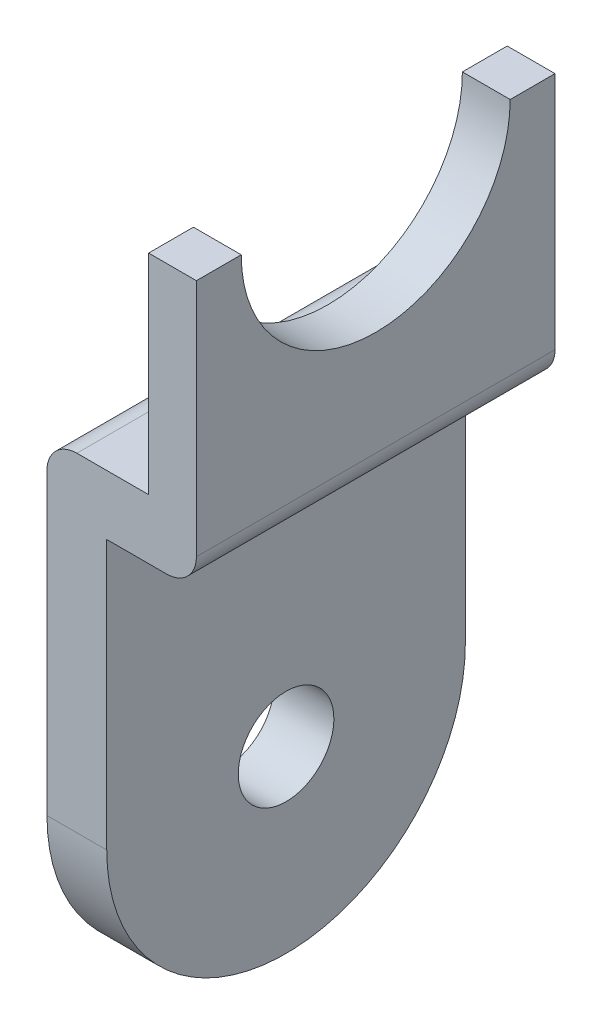
ISO-10303-21;
HEADER;
FILE_DESCRIPTION(('STEP AP214'),'2;1');
FILE_NAME('part.step','',(''),(''),'','','');
FILE_SCHEMA(('AUTOMOTIVE_DESIGN { 1 0 10303 214 1 1 1 1 }'));
ENDSEC;
DATA;
#1=APPLICATION_CONTEXT('core data for automotive mechanical design processes');
#2=APPLICATION_PROTOCOL_DEFINITION('international standard','automotive_design',2000,#1);
#3=PRODUCT_CONTEXT('',#1,'mechanical');
#4=PRODUCT('Part','Part','',(#3));
#5=PRODUCT_RELATED_PRODUCT_CATEGORY('part','',(#4));
#6=PRODUCT_DEFINITION_FORMATION('','',#4);
#7=PRODUCT_DEFINITION_CONTEXT('part definition',#1,'design');
#8=PRODUCT_DEFINITION('design','',#6,#7);
#9=PRODUCT_DEFINITION_SHAPE('','',#8);
#10=(LENGTH_UNIT() NAMED_UNIT(*) SI_UNIT(.MILLI.,.METRE.));
#11=(NAMED_UNIT(*) PLANE_ANGLE_UNIT() SI_UNIT($,.RADIAN.));
#12=(NAMED_UNIT(*) SI_UNIT($,.STERADIAN.) SOLID_ANGLE_UNIT());
#13=UNCERTAINTY_MEASURE_WITH_UNIT(LENGTH_MEASURE(1.E-05),#10,'distance_accuracy_value','');
#14=(GEOMETRIC_REPRESENTATION_CONTEXT(3) GLOBAL_UNCERTAINTY_ASSIGNED_CONTEXT((#13)) GLOBAL_UNIT_ASSIGNED_CONTEXT((#10,
#11,#12)) REPRESENTATION_CONTEXT('',''));
#15=CARTESIAN_POINT('',(0.,0.,0.));
#16=DIRECTION('',(0.,0.,1.));
#17=DIRECTION('',(1.,0.,0.));
#18=AXIS2_PLACEMENT_3D('',#15,#16,#17);
#19=CARTESIAN_POINT('',(3.4,7.,6.));
#20=DIRECTION('',(0.,-1.,0.));
#21=DIRECTION('',(0.,0.,-1.));
#22=AXIS2_PLACEMENT_3D('',#19,#20,#21);
#23=PLANE('',#22);
#24=DIRECTION('',(0.,0.,-1.));
#25=VECTOR('',#24,1.);
#26=CARTESIAN_POINT('',(3.4,7.,6.));
#27=LINE('',#26,#25);
#28=CARTESIAN_POINT('',(3.4,7.,-4.5));
#29=VERTEX_POINT('',#28);
#30=CARTESIAN_POINT('',(3.4,7.,-6.));
#31=VERTEX_POINT('',#30);
#32=EDGE_CURVE('E147',#29,#31,#27,.T.);
#33=ORIENTED_EDGE('',*,*,#32,.F.);
#34=DIRECTION('',(1.,0.,0.));
#35=VECTOR('',#34,1.);
#36=CARTESIAN_POINT('',(-0.00100000000000013,7.,-4.5));
#37=LINE('',#36,#35);
#38=CARTESIAN_POINT('',(5.,7.,-4.5));
#39=VERTEX_POINT('',#38);
#40=EDGE_CURVE('E128',#29,#39,#37,.T.);
#41=ORIENTED_EDGE('',*,*,#40,.T.);
#42=DIRECTION('',(0.,0.,-1.));
#43=VECTOR('',#42,1.);
#44=CARTESIAN_POINT('',(5.,7.,6.));
#45=LINE('',#44,#43);
#46=CARTESIAN_POINT('',(5.,7.,-6.));
#47=VERTEX_POINT('',#46);
#48=EDGE_CURVE('E144',#39,#47,#45,.T.);
#49=ORIENTED_EDGE('',*,*,#48,.T.);
#50=DIRECTION('',(-1.,0.,0.));
#51=VECTOR('',#50,1.);
#52=CARTESIAN_POINT('',(3.4,7.,-6.));
#53=LINE('',#52,#51);
#54=EDGE_CURVE('E216',#47,#31,#53,.T.);
#55=ORIENTED_EDGE('',*,*,#54,.T.);
#56=EDGE_LOOP('',(#33,#41,#49,#55));
#57=FACE_BOUND('',#56,.T.);
#58=ADVANCED_FACE('F39',(#57),#23,.F.);
#59=CARTESIAN_POINT('',(2.,-2.,6.));
#60=DIRECTION('',(-1.,0.,0.));
#61=DIRECTION('',(0.,-1.,0.));
#62=AXIS2_PLACEMENT_3D('',#59,#60,#61);
#63=PLANE('',#62);
#64=CARTESIAN_POINT('',(2.,-11.,0.));
#65=DIRECTION('',(1.,0.,0.));
#66=DIRECTION('',(0.,1.,0.));
#67=AXIS2_PLACEMENT_3D('',#64,#65,#66);
#68=CIRCLE('',#67,1.6);
#69=CARTESIAN_POINT('',(2.,-9.4,0.));
#70=VERTEX_POINT('',#69);
#71=EDGE_CURVE('E280',#70,#70,#68,.T.);
#72=ORIENTED_EDGE('',*,*,#71,.F.);
#73=EDGE_LOOP('',(#72));
#74=FACE_BOUND('',#73,.T.);
#75=DIRECTION('',(0.,1.,0.));
#76=VECTOR('',#75,1.);
#77=CARTESIAN_POINT('',(2.,-2.,6.));
#78=LINE('',#77,#76);
#79=CARTESIAN_POINT('',(2.,-11.,6.));
#80=VERTEX_POINT('',#79);
#81=CARTESIAN_POINT('',(2.,-2.,6.));
#82=VERTEX_POINT('',#81);
#83=EDGE_CURVE('E194',#80,#82,#78,.T.);
#84=ORIENTED_EDGE('',*,*,#83,.F.);
#85=CARTESIAN_POINT('',(2.,-11.,0.));
#86=DIRECTION('',(1.,0.,0.));
#87=DIRECTION('',(0.,1.,0.));
#88=AXIS2_PLACEMENT_3D('',#85,#86,#87);
#89=CIRCLE('',#88,6.);
#90=CARTESIAN_POINT('',(2.,-11.,-6.));
#91=VERTEX_POINT('',#90);
#92=EDGE_CURVE('E265',#80,#91,#89,.T.);
#93=ORIENTED_EDGE('',*,*,#92,.T.);
#94=DIRECTION('',(0.,1.,0.));
#95=VECTOR('',#94,1.);
#96=CARTESIAN_POINT('',(2.,-2.,-6.));
#97=LINE('',#96,#95);
#98=CARTESIAN_POINT('',(2.,-2.,-6.));
#99=VERTEX_POINT('',#98);
#100=EDGE_CURVE('E209',#91,#99,#97,.T.);
#101=ORIENTED_EDGE('',*,*,#100,.T.);
#102=DIRECTION('',(0.,0.,-1.));
#103=VECTOR('',#102,1.);
#104=CARTESIAN_POINT('',(2.,-2.,6.));
#105=LINE('',#104,#103);
#106=EDGE_CURVE('E156',#82,#99,#105,.T.);
#107=ORIENTED_EDGE('',*,*,#106,.F.);
#108=EDGE_LOOP('',(#84,#93,#101,#107));
#109=FACE_BOUND('',#108,.T.);
#110=ADVANCED_FACE('F229',(#74,#109),#63,.F.);
#111=CARTESIAN_POINT('',(5.,-2.,6.));
#112=DIRECTION('',(0.,1.,0.));
#113=DIRECTION('',(-1.,0.,0.));
#114=AXIS2_PLACEMENT_3D('',#111,#112,#113);
#115=PLANE('',#114);
#116=DIRECTION('',(1.,0.,0.));
#117=VECTOR('',#116,1.);
#118=CARTESIAN_POINT('',(5.,-2.,-6.));
#119=LINE('',#118,#117);
#120=CARTESIAN_POINT('',(4.,-2.,-6.));
#121=VERTEX_POINT('',#120);
#122=EDGE_CURVE('E215',#99,#121,#119,.T.);
#123=ORIENTED_EDGE('',*,*,#122,.T.);
#124=DIRECTION('',(0.,0.,-1.));
#125=VECTOR('',#124,1.);
#126=CARTESIAN_POINT('',(4.,-2.,6.));
#127=LINE('',#126,#125);
#128=CARTESIAN_POINT('',(4.,-2.,6.));
#129=VERTEX_POINT('',#128);
#130=EDGE_CURVE('E169',#121,#129,#127,.F.);
#131=ORIENTED_EDGE('',*,*,#130,.T.);
#132=DIRECTION('',(1.,0.,0.));
#133=VECTOR('',#132,1.);
#134=CARTESIAN_POINT('',(5.,-2.,6.));
#135=LINE('',#134,#133);
#136=EDGE_CURVE('E254',#82,#129,#135,.T.);
#137=ORIENTED_EDGE('',*,*,#136,.F.);
#138=ORIENTED_EDGE('',*,*,#106,.T.);
#139=EDGE_LOOP('',(#123,#131,#137,#138));
#140=FACE_BOUND('',#139,.T.);
#141=ADVANCED_FACE('F238',(#140),#115,.F.);
#142=CARTESIAN_POINT('',(5.,7.,6.));
#143=DIRECTION('',(-1.,0.,0.));
#144=DIRECTION('',(0.,-1.,0.));
#145=AXIS2_PLACEMENT_3D('',#142,#143,#144);
#146=PLANE('',#145);
#147=DIRECTION('',(0.,1.,0.));
#148=VECTOR('',#147,1.);
#149=CARTESIAN_POINT('',(5.,7.,6.));
#150=LINE('',#149,#148);
#151=CARTESIAN_POINT('',(5.,-0.999999999999999,6.));
#152=VERTEX_POINT('',#151);
#153=CARTESIAN_POINT('',(5.,7.,6.));
#154=VERTEX_POINT('',#153);
#155=EDGE_CURVE('E252',#152,#154,#150,.T.);
#156=ORIENTED_EDGE('',*,*,#155,.F.);
#157=DIRECTION('',(0.,0.,-1.));
#158=VECTOR('',#157,1.);
#159=CARTESIAN_POINT('',(5.,-0.999999999999999,6.));
#160=LINE('',#159,#158);
#161=CARTESIAN_POINT('',(5.,-0.999999999999999,-6.));
#162=VERTEX_POINT('',#161);
#163=EDGE_CURVE('E161',#152,#162,#160,.T.);
#164=ORIENTED_EDGE('',*,*,#163,.T.);
#165=DIRECTION('',(0.,1.,0.));
#166=VECTOR('',#165,1.);
#167=CARTESIAN_POINT('',(5.,7.,-6.));
#168=LINE('',#167,#166);
#169=EDGE_CURVE('E152',#162,#47,#168,.T.);
#170=ORIENTED_EDGE('',*,*,#169,.T.);
#171=ORIENTED_EDGE('',*,*,#48,.F.);
#172=CARTESIAN_POINT('',(5.,7.,0.));
#173=DIRECTION('',(1.,0.,0.));
#174=DIRECTION('',(0.,1.,0.));
#175=AXIS2_PLACEMENT_3D('',#172,#173,#174);
#176=CIRCLE('',#175,4.5);
#177=CARTESIAN_POINT('',(5.,7.,4.5));
#178=VERTEX_POINT('',#177);
#179=EDGE_CURVE('E130',#178,#39,#176,.T.);
#180=ORIENTED_EDGE('',*,*,#179,.F.);
#181=EDGE_CURVE('E154',#154,#178,#45,.T.);
#182=ORIENTED_EDGE('',*,*,#181,.F.);
#183=EDGE_LOOP('',(#156,#164,#170,#171,#180,#182));
#184=FACE_BOUND('',#183,.T.);
#185=ADVANCED_FACE('F146',(#184),#146,.F.);
#186=ORIENTED_EDGE('',*,*,#181,.T.);
#187=DIRECTION('',(1.,0.,0.));
#188=VECTOR('',#187,1.);
#189=CARTESIAN_POINT('',(-0.00100000000000013,7.,4.5));
#190=LINE('',#189,#188);
#191=CARTESIAN_POINT('',(3.4,7.,4.5));
#192=VERTEX_POINT('',#191);
#193=EDGE_CURVE('E134',#192,#178,#190,.T.);
#194=ORIENTED_EDGE('',*,*,#193,.F.);
#195=CARTESIAN_POINT('',(3.4,7.,6.));
#196=VERTEX_POINT('',#195);
#197=EDGE_CURVE('E153',#196,#192,#27,.T.);
#198=ORIENTED_EDGE('',*,*,#197,.F.);
#199=DIRECTION('',(-1.,0.,0.));
#200=VECTOR('',#199,1.);
#201=CARTESIAN_POINT('',(3.4,7.,6.));
#202=LINE('',#201,#200);
#203=EDGE_CURVE('E249',#154,#196,#202,.T.);
#204=ORIENTED_EDGE('',*,*,#203,.F.);
#205=EDGE_LOOP('',(#186,#194,#198,#204));
#206=FACE_BOUND('',#205,.T.);
#207=ADVANCED_FACE('F235',(#206),#23,.F.);
#208=CARTESIAN_POINT('',(3.4,0.,6.));
#209=DIRECTION('',(1.,0.,0.));
#210=DIRECTION('',(0.,1.,0.));
#211=AXIS2_PLACEMENT_3D('',#208,#209,#210);
#212=PLANE('',#211);
#213=ORIENTED_EDGE('',*,*,#197,.T.);
#214=CARTESIAN_POINT('',(3.4,7.,0.));
#215=DIRECTION('',(1.,0.,0.));
#216=DIRECTION('',(0.,1.,0.));
#217=AXIS2_PLACEMENT_3D('',#214,#215,#216);
#218=CIRCLE('',#217,4.5);
#219=EDGE_CURVE('E139',#29,#192,#218,.F.);
#220=ORIENTED_EDGE('',*,*,#219,.F.);
#221=ORIENTED_EDGE('',*,*,#32,.T.);
#222=DIRECTION('',(0.,-1.,0.));
#223=VECTOR('',#222,1.);
#224=CARTESIAN_POINT('',(3.4,0.,-6.));
#225=LINE('',#224,#223);
#226=CARTESIAN_POINT('',(3.4,0.,-6.));
#227=VERTEX_POINT('',#226);
#228=EDGE_CURVE('E193',#31,#227,#225,.T.);
#229=ORIENTED_EDGE('',*,*,#228,.T.);
#230=DIRECTION('',(0.,0.,-1.));
#231=VECTOR('',#230,1.);
#232=CARTESIAN_POINT('',(3.4,0.,6.));
#233=LINE('',#232,#231);
#234=CARTESIAN_POINT('',(3.4,0.,6.));
#235=VERTEX_POINT('',#234);
#236=EDGE_CURVE('E199',#235,#227,#233,.T.);
#237=ORIENTED_EDGE('',*,*,#236,.F.);
#238=DIRECTION('',(0.,-1.,0.));
#239=VECTOR('',#238,1.);
#240=CARTESIAN_POINT('',(3.4,0.,6.));
#241=LINE('',#240,#239);
#242=EDGE_CURVE('E203',#196,#235,#241,.T.);
#243=ORIENTED_EDGE('',*,*,#242,.F.);
#244=EDGE_LOOP('',(#213,#220,#221,#229,#237,#243));
#245=FACE_BOUND('',#244,.T.);
#246=ADVANCED_FACE('F218',(#245),#212,.F.);
#247=CARTESIAN_POINT('',(0.,0.,6.));
#248=DIRECTION('',(0.,-1.,0.));
#249=DIRECTION('',(0.,0.,-1.));
#250=AXIS2_PLACEMENT_3D('',#247,#248,#249);
#251=PLANE('',#250);
#252=DIRECTION('',(-1.,0.,0.));
#253=VECTOR('',#252,1.);
#254=CARTESIAN_POINT('',(0.,0.,-6.));
#255=LINE('',#254,#253);
#256=CARTESIAN_POINT('',(1.,0.,-6.));
#257=VERTEX_POINT('',#256);
#258=EDGE_CURVE('E188',#227,#257,#255,.T.);
#259=ORIENTED_EDGE('',*,*,#258,.T.);
#260=DIRECTION('',(0.,0.,-1.));
#261=VECTOR('',#260,1.);
#262=CARTESIAN_POINT('',(1.,0.,6.));
#263=LINE('',#262,#261);
#264=CARTESIAN_POINT('',(1.,0.,6.));
#265=VERTEX_POINT('',#264);
#266=EDGE_CURVE('E11',#257,#265,#263,.F.);
#267=ORIENTED_EDGE('',*,*,#266,.T.);
#268=DIRECTION('',(-1.,0.,0.));
#269=VECTOR('',#268,1.);
#270=CARTESIAN_POINT('',(0.,0.,6.));
#271=LINE('',#270,#269);
#272=EDGE_CURVE('E201',#235,#265,#271,.T.);
#273=ORIENTED_EDGE('',*,*,#272,.F.);
#274=ORIENTED_EDGE('',*,*,#236,.T.);
#275=EDGE_LOOP('',(#259,#267,#273,#274));
#276=FACE_BOUND('',#275,.T.);
#277=ADVANCED_FACE('F221',(#276),#251,.F.);
#278=CARTESIAN_POINT('',(0.,-11.,6.));
#279=DIRECTION('',(1.,0.,0.));
#280=DIRECTION('',(0.,0.,-1.));
#281=AXIS2_PLACEMENT_3D('',#278,#279,#280);
#282=PLANE('',#281);
#283=CARTESIAN_POINT('',(0.,-11.,0.));
#284=DIRECTION('',(1.,0.,0.));
#285=DIRECTION('',(0.,0.,-1.));
#286=AXIS2_PLACEMENT_3D('',#283,#284,#285);
#287=CIRCLE('',#286,1.6);
#288=CARTESIAN_POINT('',(0.,-11.,-1.6));
#289=VERTEX_POINT('',#288);
#290=EDGE_CURVE('E274',#289,#289,#287,.F.);
#291=ORIENTED_EDGE('',*,*,#290,.F.);
#292=EDGE_LOOP('',(#291));
#293=FACE_BOUND('',#292,.T.);
#294=DIRECTION('',(0.,-1.,0.));
#295=VECTOR('',#294,1.);
#296=CARTESIAN_POINT('',(0.,-11.,6.));
#297=LINE('',#296,#295);
#298=CARTESIAN_POINT('',(0.,-0.999999999999999,6.));
#299=VERTEX_POINT('',#298);
#300=CARTESIAN_POINT('',(0.,-11.,6.));
#301=VERTEX_POINT('',#300);
#302=EDGE_CURVE('E181',#299,#301,#297,.T.);
#303=ORIENTED_EDGE('',*,*,#302,.F.);
#304=DIRECTION('',(0.,0.,-1.));
#305=VECTOR('',#304,1.);
#306=CARTESIAN_POINT('',(0.,-0.999999999999999,6.));
#307=LINE('',#306,#305);
#308=CARTESIAN_POINT('',(0.,-0.999999999999999,-6.));
#309=VERTEX_POINT('',#308);
#310=EDGE_CURVE('E50',#299,#309,#307,.T.);
#311=ORIENTED_EDGE('',*,*,#310,.T.);
#312=DIRECTION('',(0.,-1.,0.));
#313=VECTOR('',#312,1.);
#314=CARTESIAN_POINT('',(0.,-11.,-6.));
#315=LINE('',#314,#313);
#316=CARTESIAN_POINT('',(0.,-11.,-6.));
#317=VERTEX_POINT('',#316);
#318=EDGE_CURVE('E177',#309,#317,#315,.T.);
#319=ORIENTED_EDGE('',*,*,#318,.T.);
#320=CARTESIAN_POINT('',(0.,-11.,0.));
#321=DIRECTION('',(1.,0.,0.));
#322=DIRECTION('',(0.,0.,-1.));
#323=AXIS2_PLACEMENT_3D('',#320,#321,#322);
#324=CIRCLE('',#323,6.);
#325=EDGE_CURVE('E208',#317,#301,#324,.F.);
#326=ORIENTED_EDGE('',*,*,#325,.T.);
#327=EDGE_LOOP('',(#303,#311,#319,#326));
#328=FACE_BOUND('',#327,.T.);
#329=ADVANCED_FACE('F180',(#293,#328),#282,.F.);
#330=CARTESIAN_POINT('',(0.,0.,6.));
#331=DIRECTION('',(0.,0.,-1.));
#332=DIRECTION('',(-1.,0.,0.));
#333=AXIS2_PLACEMENT_3D('',#330,#331,#332);
#334=PLANE('',#333);
#335=ORIENTED_EDGE('',*,*,#136,.T.);
#336=CARTESIAN_POINT('',(4.,-0.999999999999999,6.));
#337=DIRECTION('',(0.,0.,-1.));
#338=DIRECTION('',(-1.,0.,0.));
#339=AXIS2_PLACEMENT_3D('',#336,#337,#338);
#340=CIRCLE('',#339,1.);
#341=EDGE_CURVE('E175',#129,#152,#340,.F.);
#342=ORIENTED_EDGE('',*,*,#341,.T.);
#343=ORIENTED_EDGE('',*,*,#155,.T.);
#344=ORIENTED_EDGE('',*,*,#203,.T.);
#345=ORIENTED_EDGE('',*,*,#242,.T.);
#346=ORIENTED_EDGE('',*,*,#272,.T.);
#347=CARTESIAN_POINT('',(1.,-0.999999999999999,6.));
#348=DIRECTION('',(0.,0.,-1.));
#349=DIRECTION('',(-1.,0.,0.));
#350=AXIS2_PLACEMENT_3D('',#347,#348,#349);
#351=CIRCLE('',#350,1.);
#352=EDGE_CURVE('E53',#265,#299,#351,.F.);
#353=ORIENTED_EDGE('',*,*,#352,.T.);
#354=ORIENTED_EDGE('',*,*,#302,.T.);
#355=DIRECTION('',(1.,0.,0.));
#356=VECTOR('',#355,1.);
#357=CARTESIAN_POINT('',(2.,-11.,6.));
#358=LINE('',#357,#356);
#359=EDGE_CURVE('E186',#301,#80,#358,.T.);
#360=ORIENTED_EDGE('',*,*,#359,.T.);
#361=ORIENTED_EDGE('',*,*,#83,.T.);
#362=EDGE_LOOP('',(#335,#342,#343,#344,#345,#346,#353,#354,#360,#361));
#363=FACE_BOUND('',#362,.T.);
#364=ADVANCED_FACE('F271',(#363),#334,.F.);
#365=CARTESIAN_POINT('',(0.,0.,-6.));
#366=DIRECTION('',(0.,0.,-1.));
#367=DIRECTION('',(-1.,0.,0.));
#368=AXIS2_PLACEMENT_3D('',#365,#366,#367);
#369=PLANE('',#368);
#370=ORIENTED_EDGE('',*,*,#169,.F.);
#371=CARTESIAN_POINT('',(4.,-0.999999999999999,-6.));
#372=DIRECTION('',(0.,0.,-1.));
#373=DIRECTION('',(-1.,0.,0.));
#374=AXIS2_PLACEMENT_3D('',#371,#372,#373);
#375=CIRCLE('',#374,1.);
#376=EDGE_CURVE('E170',#162,#121,#375,.T.);
#377=ORIENTED_EDGE('',*,*,#376,.T.);
#378=ORIENTED_EDGE('',*,*,#122,.F.);
#379=ORIENTED_EDGE('',*,*,#100,.F.);
#380=DIRECTION('',(1.,0.,0.));
#381=VECTOR('',#380,1.);
#382=CARTESIAN_POINT('',(2.,-11.,-6.));
#383=LINE('',#382,#381);
#384=EDGE_CURVE('E190',#317,#91,#383,.T.);
#385=ORIENTED_EDGE('',*,*,#384,.F.);
#386=ORIENTED_EDGE('',*,*,#318,.F.);
#387=CARTESIAN_POINT('',(1.,-0.999999999999999,-6.));
#388=DIRECTION('',(0.,0.,-1.));
#389=DIRECTION('',(-1.,0.,0.));
#390=AXIS2_PLACEMENT_3D('',#387,#388,#389);
#391=CIRCLE('',#390,1.);
#392=EDGE_CURVE('E164',#309,#257,#391,.T.);
#393=ORIENTED_EDGE('',*,*,#392,.T.);
#394=ORIENTED_EDGE('',*,*,#258,.F.);
#395=ORIENTED_EDGE('',*,*,#228,.F.);
#396=ORIENTED_EDGE('',*,*,#54,.F.);
#397=EDGE_LOOP('',(#370,#377,#378,#379,#385,#386,#393,#394,#395,#396));
#398=FACE_BOUND('',#397,.T.);
#399=ADVANCED_FACE('F183',(#398),#369,.T.);
#400=CARTESIAN_POINT('',(-16.9705627484771,-11.,0.));
#401=DIRECTION('',(1.,0.,0.));
#402=DIRECTION('',(0.,1.,0.));
#403=AXIS2_PLACEMENT_3D('',#400,#401,#402);
#404=CYLINDRICAL_SURFACE('',#403,6.);
#405=ORIENTED_EDGE('',*,*,#359,.F.);
#406=ORIENTED_EDGE('',*,*,#325,.F.);
#407=ORIENTED_EDGE('',*,*,#384,.T.);
#408=ORIENTED_EDGE('',*,*,#92,.F.);
#409=EDGE_LOOP('',(#405,#406,#407,#408));
#410=FACE_BOUND('',#409,.T.);
#411=ADVANCED_FACE('F267',(#410),#404,.T.);
#412=CARTESIAN_POINT('',(-0.00100000000000013,7.,0.));
#413=DIRECTION('',(1.,0.,0.));
#414=DIRECTION('',(0.,1.,0.));
#415=AXIS2_PLACEMENT_3D('',#412,#413,#414);
#416=CYLINDRICAL_SURFACE('',#415,4.5);
#417=ORIENTED_EDGE('',*,*,#219,.T.);
#418=ORIENTED_EDGE('',*,*,#193,.T.);
#419=ORIENTED_EDGE('',*,*,#179,.T.);
#420=ORIENTED_EDGE('',*,*,#40,.F.);
#421=EDGE_LOOP('',(#417,#418,#419,#420));
#422=FACE_BOUND('',#421,.T.);
#423=ADVANCED_FACE('F126',(#422),#416,.F.);
#424=CARTESIAN_POINT('',(-0.00100000000000057,-11.,0.));
#425=DIRECTION('',(1.,0.,0.));
#426=DIRECTION('',(0.,1.,0.));
#427=AXIS2_PLACEMENT_3D('',#424,#425,#426);
#428=CYLINDRICAL_SURFACE('',#427,1.6);
#429=ORIENTED_EDGE('',*,*,#71,.T.);
#430=EDGE_LOOP('',(#429));
#431=FACE_BOUND('',#430,.T.);
#432=ORIENTED_EDGE('',*,*,#290,.T.);
#433=EDGE_LOOP('',(#432));
#434=FACE_BOUND('',#433,.T.);
#435=ADVANCED_FACE('F227',(#431,#434),#428,.F.);
#436=CARTESIAN_POINT('',(4.,-0.999999999999999,6.));
#437=DIRECTION('',(0.,0.,-1.));
#438=DIRECTION('',(-1.,0.,0.));
#439=AXIS2_PLACEMENT_3D('',#436,#437,#438);
#440=CYLINDRICAL_SURFACE('',#439,1.);
#441=ORIENTED_EDGE('',*,*,#341,.F.);
#442=ORIENTED_EDGE('',*,*,#130,.F.);
#443=ORIENTED_EDGE('',*,*,#376,.F.);
#444=ORIENTED_EDGE('',*,*,#163,.F.);
#445=EDGE_LOOP('',(#441,#442,#443,#444));
#446=FACE_BOUND('',#445,.T.);
#447=ADVANCED_FACE('F224',(#446),#440,.T.);
#448=CARTESIAN_POINT('',(1.,-0.999999999999999,6.));
#449=DIRECTION('',(0.,0.,-1.));
#450=DIRECTION('',(-1.,0.,0.));
#451=AXIS2_PLACEMENT_3D('',#448,#449,#450);
#452=CYLINDRICAL_SURFACE('',#451,1.);
#453=ORIENTED_EDGE('',*,*,#352,.F.);
#454=ORIENTED_EDGE('',*,*,#266,.F.);
#455=ORIENTED_EDGE('',*,*,#392,.F.);
#456=ORIENTED_EDGE('',*,*,#310,.F.);
#457=EDGE_LOOP('',(#453,#454,#455,#456));
#458=FACE_BOUND('',#457,.T.);
#459=ADVANCED_FACE('F41',(#458),#452,.T.);
#460=CLOSED_SHELL('',(#58,#110,#141,#185,#207,#246,#277,#329,#364,#399,#411,#423,#435,#447,#459));
#461=MANIFOLD_SOLID_BREP('B2',#460);
#462=ADVANCED_BREP_SHAPE_REPRESENTATION('',(#18,#461),#14);
#463=SHAPE_DEFINITION_REPRESENTATION(#9,#462);
ENDSEC;
END-ISO-10303-21;
